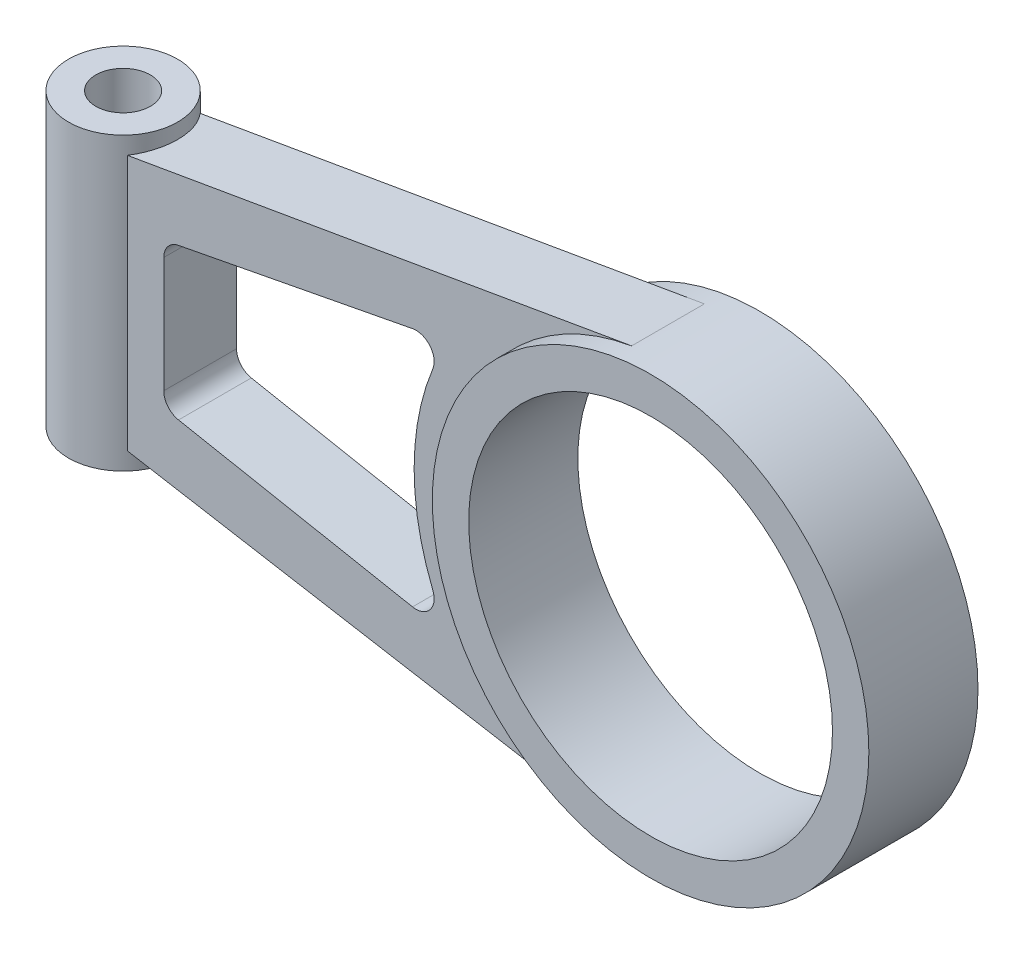
ISO-10303-21;
HEADER;
FILE_DESCRIPTION(('STEP AP214'),'2;1');
FILE_NAME('part.step','',(''),(''),'','','');
FILE_SCHEMA(('AUTOMOTIVE_DESIGN { 1 0 10303 214 1 1 1 1 }'));
ENDSEC;
DATA;
#1=APPLICATION_CONTEXT('core data for automotive mechanical design processes');
#2=APPLICATION_PROTOCOL_DEFINITION('international standard','automotive_design',2000,#1);
#3=PRODUCT_CONTEXT('',#1,'mechanical');
#4=PRODUCT('Part','Part','',(#3));
#5=PRODUCT_RELATED_PRODUCT_CATEGORY('part','',(#4));
#6=PRODUCT_DEFINITION_FORMATION('','',#4);
#7=PRODUCT_DEFINITION_CONTEXT('part definition',#1,'design');
#8=PRODUCT_DEFINITION('design','',#6,#7);
#9=PRODUCT_DEFINITION_SHAPE('','',#8);
#10=(LENGTH_UNIT() NAMED_UNIT(*) SI_UNIT(.MILLI.,.METRE.));
#11=(NAMED_UNIT(*) PLANE_ANGLE_UNIT() SI_UNIT($,.RADIAN.));
#12=(NAMED_UNIT(*) SI_UNIT($,.STERADIAN.) SOLID_ANGLE_UNIT());
#13=UNCERTAINTY_MEASURE_WITH_UNIT(LENGTH_MEASURE(1.E-05),#10,'distance_accuracy_value','');
#14=(GEOMETRIC_REPRESENTATION_CONTEXT(3) GLOBAL_UNCERTAINTY_ASSIGNED_CONTEXT((#13)) GLOBAL_UNIT_ASSIGNED_CONTEXT((#10,
#11,#12)) REPRESENTATION_CONTEXT('',''));
#15=CARTESIAN_POINT('',(0.,0.,0.));
#16=DIRECTION('',(0.,0.,1.));
#17=DIRECTION('',(1.,0.,0.));
#18=AXIS2_PLACEMENT_3D('',#15,#16,#17);
#19=CARTESIAN_POINT('',(0.,0.,10.));
#20=DIRECTION('',(0.,0.,1.));
#21=DIRECTION('',(1.,0.,0.));
#22=AXIS2_PLACEMENT_3D('',#19,#20,#21);
#23=PLANE('',#22);
#24=CARTESIAN_POINT('',(-133.819660112501,15.8679479378662,9.99999999999999));
#25=DIRECTION('',(0.,0.,1.));
#26=DIRECTION('',(1.,0.,0.));
#27=AXIS2_PLACEMENT_3D('',#24,#25,#26);
#28=CIRCLE('',#27,5.);
#29=CARTESIAN_POINT('',(-134.761592566539,20.77842278782,9.99999999999999));
#30=VERTEX_POINT('',#29);
#31=CARTESIAN_POINT('',(-138.819660112501,15.8679479378662,10.));
#32=VERTEX_POINT('',#31);
#33=EDGE_CURVE('E139',#30,#32,#28,.T.);
#34=ORIENTED_EDGE('',*,*,#33,.F.);
#35=DIRECTION('',(-0.982094969990767,-0.188386490807685,0.));
#36=VECTOR('',#35,1.);
#37=CARTESIAN_POINT('',(-8.62690465243416,44.9737113814315,10.));
#38=LINE('',#37,#36);
#39=CARTESIAN_POINT('',(-70.4355513802943,33.11751171192,9.99999999999999));
#40=VERTEX_POINT('',#39);
#41=EDGE_CURVE('E216',#40,#30,#38,.T.);
#42=ORIENTED_EDGE('',*,*,#41,.F.);
#43=CARTESIAN_POINT('',(-69.4936189262559,28.2070368619661,9.99999999999999));
#44=DIRECTION('',(0.,0.,1.));
#45=DIRECTION('',(1.,0.,0.));
#46=AXIS2_PLACEMENT_3D('',#43,#44,#45);
#47=CIRCLE('',#46,5.);
#48=CARTESIAN_POINT('',(-64.8607109978388,26.3265677378351,9.99999999999999));
#49=VERTEX_POINT('',#48);
#50=EDGE_CURVE('E217',#49,#40,#47,.T.);
#51=ORIENTED_EDGE('',*,*,#50,.F.);
#52=CARTESIAN_POINT('',(0.,0.,9.99999999999999));
#53=DIRECTION('',(0.,0.,1.));
#54=DIRECTION('',(1.,0.,0.));
#55=AXIS2_PLACEMENT_3D('',#52,#53,#54);
#56=CIRCLE('',#55,69.9999999999997);
#57=CARTESIAN_POINT('',(-64.8607109978386,-26.3265677378351,9.99999999999999));
#58=VERTEX_POINT('',#57);
#59=EDGE_CURVE('E219',#58,#49,#56,.F.);
#60=ORIENTED_EDGE('',*,*,#59,.F.);
#61=CARTESIAN_POINT('',(-69.4936189262554,-28.2070368619662,9.99999999999999));
#62=DIRECTION('',(0.,0.,1.));
#63=DIRECTION('',(1.,0.,0.));
#64=AXIS2_PLACEMENT_3D('',#61,#62,#63);
#65=CIRCLE('',#64,5.);
#66=CARTESIAN_POINT('',(-70.4355513802939,-33.11751171192,9.99999999999999));
#67=VERTEX_POINT('',#66);
#68=EDGE_CURVE('E225',#67,#58,#65,.T.);
#69=ORIENTED_EDGE('',*,*,#68,.F.);
#70=DIRECTION('',(0.982094969990768,-0.188386490807683,0.));
#71=VECTOR('',#70,1.);
#72=CARTESIAN_POINT('',(-8.62690465243404,-44.9737113814314,10.));
#73=LINE('',#72,#71);
#74=CARTESIAN_POINT('',(-134.761592566539,-20.7784227878201,9.99999999999999));
#75=VERTEX_POINT('',#74);
#76=EDGE_CURVE('E221',#75,#67,#73,.T.);
#77=ORIENTED_EDGE('',*,*,#76,.F.);
#78=CARTESIAN_POINT('',(-133.819660112501,-15.8679479378662,9.99999999999999));
#79=DIRECTION('',(0.,0.,1.));
#80=DIRECTION('',(1.,0.,0.));
#81=AXIS2_PLACEMENT_3D('',#78,#79,#80);
#82=CIRCLE('',#81,5.);
#83=CARTESIAN_POINT('',(-138.819660112501,-15.8679479378662,9.99999999999999));
#84=VERTEX_POINT('',#83);
#85=EDGE_CURVE('E226',#84,#75,#82,.T.);
#86=ORIENTED_EDGE('',*,*,#85,.F.);
#87=DIRECTION('',(0.,-1.,0.));
#88=VECTOR('',#87,1.);
#89=CARTESIAN_POINT('',(-138.819660112501,0.,10.));
#90=LINE('',#89,#88);
#91=EDGE_CURVE('E229',#32,#84,#90,.T.);
#92=ORIENTED_EDGE('',*,*,#91,.F.);
#93=EDGE_LOOP('',(#34,#42,#51,#60,#69,#77,#86,#92));
#94=FACE_BOUND('',#93,.T.);
#95=DIRECTION('',(-0.985406838508122,-0.170215635654975,0.));
#96=VECTOR('',#95,1.);
#97=CARTESIAN_POINT('',(-10.2129381392985,59.1244103104874,10.));
#98=LINE('',#97,#96);
#99=CARTESIAN_POINT('',(-10.2129381392985,59.1244103104874,10.));
#100=VERTEX_POINT('',#99);
#101=CARTESIAN_POINT('',(-148.819660112501,35.1819833201893,10.));
#102=VERTEX_POINT('',#101);
#103=EDGE_CURVE('E179',#100,#102,#98,.T.);
#104=ORIENTED_EDGE('',*,*,#103,.T.);
#105=DIRECTION('',(0.,-1.,0.));
#106=VECTOR('',#105,1.);
#107=CARTESIAN_POINT('',(-148.819660112501,40.,10.));
#108=LINE('',#107,#106);
#109=CARTESIAN_POINT('',(-148.819660112501,-35.1819833201894,10.));
#110=VERTEX_POINT('',#109);
#111=EDGE_CURVE('E188',#102,#110,#108,.T.);
#112=ORIENTED_EDGE('',*,*,#111,.T.);
#113=DIRECTION('',(-0.985406838508122,0.170215635654975,0.));
#114=VECTOR('',#113,1.);
#115=CARTESIAN_POINT('',(-10.2129381392985,-59.1244103104874,10.));
#116=LINE('',#115,#114);
#117=CARTESIAN_POINT('',(-10.2129381392985,-59.1244103104873,10.));
#118=VERTEX_POINT('',#117);
#119=EDGE_CURVE('E194',#118,#110,#116,.T.);
#120=ORIENTED_EDGE('',*,*,#119,.F.);
#121=CARTESIAN_POINT('',(0.,0.,10.));
#122=DIRECTION('',(0.,0.,1.));
#123=DIRECTION('',(1.,0.,0.));
#124=AXIS2_PLACEMENT_3D('',#121,#122,#123);
#125=CIRCLE('',#124,60.);
#126=EDGE_CURVE('E181',#100,#118,#125,.T.);
#127=ORIENTED_EDGE('',*,*,#126,.F.);
#128=EDGE_LOOP('',(#104,#112,#120,#127));
#129=FACE_BOUND('',#128,.T.);
#130=ADVANCED_FACE('F39',(#94,#129),#23,.T.);
#131=CARTESIAN_POINT('',(0.,0.,-10.));
#132=DIRECTION('',(0.,0.,1.));
#133=DIRECTION('',(1.,0.,0.));
#134=AXIS2_PLACEMENT_3D('',#131,#132,#133);
#135=PLANE('',#134);
#136=DIRECTION('',(-0.982094969990767,-0.188386490807685,0.));
#137=VECTOR('',#136,1.);
#138=CARTESIAN_POINT('',(-8.62690465243416,44.9737113814315,-10.));
#139=LINE('',#138,#137);
#140=CARTESIAN_POINT('',(-70.4355513802943,33.11751171192,-9.99999999999999));
#141=VERTEX_POINT('',#140);
#142=CARTESIAN_POINT('',(-134.761592566539,20.77842278782,-9.99999999999999));
#143=VERTEX_POINT('',#142);
#144=EDGE_CURVE('E50',#141,#143,#139,.T.);
#145=ORIENTED_EDGE('',*,*,#144,.T.);
#146=CARTESIAN_POINT('',(-133.819660112501,15.8679479378662,-9.99999999999999));
#147=DIRECTION('',(0.,0.,1.));
#148=DIRECTION('',(1.,0.,0.));
#149=AXIS2_PLACEMENT_3D('',#146,#147,#148);
#150=CIRCLE('',#149,5.);
#151=CARTESIAN_POINT('',(-138.819660112501,15.8679479378662,-9.99999999999999));
#152=VERTEX_POINT('',#151);
#153=EDGE_CURVE('E11',#143,#152,#150,.T.);
#154=ORIENTED_EDGE('',*,*,#153,.T.);
#155=DIRECTION('',(0.,-1.,0.));
#156=VECTOR('',#155,1.);
#157=CARTESIAN_POINT('',(-138.819660112501,0.,-10.));
#158=LINE('',#157,#156);
#159=CARTESIAN_POINT('',(-138.819660112501,-15.8679479378662,-10.));
#160=VERTEX_POINT('',#159);
#161=EDGE_CURVE('E123',#152,#160,#158,.T.);
#162=ORIENTED_EDGE('',*,*,#161,.T.);
#163=CARTESIAN_POINT('',(-133.819660112501,-15.8679479378662,-9.99999999999999));
#164=DIRECTION('',(0.,0.,1.));
#165=DIRECTION('',(1.,0.,0.));
#166=AXIS2_PLACEMENT_3D('',#163,#164,#165);
#167=CIRCLE('',#166,5.);
#168=CARTESIAN_POINT('',(-134.761592566539,-20.7784227878201,-9.99999999999999));
#169=VERTEX_POINT('',#168);
#170=EDGE_CURVE('E129',#160,#169,#167,.T.);
#171=ORIENTED_EDGE('',*,*,#170,.T.);
#172=DIRECTION('',(0.982094969990768,-0.188386490807683,0.));
#173=VECTOR('',#172,1.);
#174=CARTESIAN_POINT('',(-8.62690465243404,-44.9737113814314,-10.));
#175=LINE('',#174,#173);
#176=CARTESIAN_POINT('',(-70.4355513802939,-33.11751171192,-9.99999999999999));
#177=VERTEX_POINT('',#176);
#178=EDGE_CURVE('E156',#169,#177,#175,.T.);
#179=ORIENTED_EDGE('',*,*,#178,.T.);
#180=CARTESIAN_POINT('',(-69.4936189262554,-28.2070368619662,-9.99999999999999));
#181=DIRECTION('',(0.,0.,1.));
#182=DIRECTION('',(1.,0.,0.));
#183=AXIS2_PLACEMENT_3D('',#180,#181,#182);
#184=CIRCLE('',#183,5.);
#185=CARTESIAN_POINT('',(-64.8607109978386,-26.3265677378351,-9.99999999999999));
#186=VERTEX_POINT('',#185);
#187=EDGE_CURVE('E153',#177,#186,#184,.T.);
#188=ORIENTED_EDGE('',*,*,#187,.T.);
#189=CARTESIAN_POINT('',(0.,0.,-9.99999999999999));
#190=DIRECTION('',(0.,0.,1.));
#191=DIRECTION('',(1.,0.,0.));
#192=AXIS2_PLACEMENT_3D('',#189,#190,#191);
#193=CIRCLE('',#192,69.9999999999997);
#194=CARTESIAN_POINT('',(-64.8607109978388,26.3265677378351,-9.99999999999999));
#195=VERTEX_POINT('',#194);
#196=EDGE_CURVE('E149',#186,#195,#193,.F.);
#197=ORIENTED_EDGE('',*,*,#196,.T.);
#198=CARTESIAN_POINT('',(-69.4936189262559,28.2070368619661,-9.99999999999999));
#199=DIRECTION('',(0.,0.,1.));
#200=DIRECTION('',(1.,0.,0.));
#201=AXIS2_PLACEMENT_3D('',#198,#199,#200);
#202=CIRCLE('',#201,5.);
#203=EDGE_CURVE('E144',#195,#141,#202,.T.);
#204=ORIENTED_EDGE('',*,*,#203,.T.);
#205=EDGE_LOOP('',(#145,#154,#162,#171,#179,#188,#197,#204));
#206=FACE_BOUND('',#205,.T.);
#207=DIRECTION('',(0.,-1.,0.));
#208=VECTOR('',#207,1.);
#209=CARTESIAN_POINT('',(-148.819660112501,40.,-10.));
#210=LINE('',#209,#208);
#211=CARTESIAN_POINT('',(-148.819660112501,35.1819833201893,-10.));
#212=VERTEX_POINT('',#211);
#213=CARTESIAN_POINT('',(-148.819660112501,-35.1819833201894,-10.));
#214=VERTEX_POINT('',#213);
#215=EDGE_CURVE('E128',#212,#214,#210,.T.);
#216=ORIENTED_EDGE('',*,*,#215,.F.);
#217=DIRECTION('',(-0.985406838508122,-0.170215635654975,0.));
#218=VECTOR('',#217,1.);
#219=CARTESIAN_POINT('',(-10.2129381392985,59.1244103104874,-10.));
#220=LINE('',#219,#218);
#221=CARTESIAN_POINT('',(-10.2129381392985,59.1244103104873,-10.));
#222=VERTEX_POINT('',#221);
#223=EDGE_CURVE('E178',#222,#212,#220,.T.);
#224=ORIENTED_EDGE('',*,*,#223,.F.);
#225=CARTESIAN_POINT('',(0.,0.,-10.));
#226=DIRECTION('',(0.,0.,1.));
#227=DIRECTION('',(1.,0.,0.));
#228=AXIS2_PLACEMENT_3D('',#225,#226,#227);
#229=CIRCLE('',#228,60.);
#230=CARTESIAN_POINT('',(-10.2129381392985,-59.1244103104874,-10.));
#231=VERTEX_POINT('',#230);
#232=EDGE_CURVE('E186',#222,#231,#229,.T.);
#233=ORIENTED_EDGE('',*,*,#232,.T.);
#234=DIRECTION('',(-0.985406838508122,0.170215635654975,0.));
#235=VECTOR('',#234,1.);
#236=CARTESIAN_POINT('',(-10.2129381392985,-59.1244103104874,-10.));
#237=LINE('',#236,#235);
#238=EDGE_CURVE('E184',#231,#214,#237,.T.);
#239=ORIENTED_EDGE('',*,*,#238,.T.);
#240=EDGE_LOOP('',(#216,#224,#233,#239));
#241=FACE_BOUND('',#240,.T.);
#242=ADVANCED_FACE('F143',(#206,#241),#135,.F.);
#243=CARTESIAN_POINT('',(0.,0.,15.));
#244=DIRECTION('',(0.,0.,1.));
#245=DIRECTION('',(1.,0.,0.));
#246=AXIS2_PLACEMENT_3D('',#243,#244,#245);
#247=PLANE('',#246);
#248=CARTESIAN_POINT('',(0.,0.,15.));
#249=DIRECTION('',(0.,0.,1.));
#250=DIRECTION('',(1.,0.,0.));
#251=AXIS2_PLACEMENT_3D('',#248,#249,#250);
#252=CIRCLE('',#251,60.);
#253=CARTESIAN_POINT('',(60.,0.,15.));
#254=VERTEX_POINT('',#253);
#255=EDGE_CURVE('E165',#254,#254,#252,.T.);
#256=ORIENTED_EDGE('',*,*,#255,.T.);
#257=EDGE_LOOP('',(#256));
#258=FACE_BOUND('',#257,.T.);
#259=CARTESIAN_POINT('',(0.,0.,15.));
#260=DIRECTION('',(0.,0.,1.));
#261=DIRECTION('',(1.,0.,0.));
#262=AXIS2_PLACEMENT_3D('',#259,#260,#261);
#263=CIRCLE('',#262,50.);
#264=CARTESIAN_POINT('',(50.,0.,15.));
#265=VERTEX_POINT('',#264);
#266=EDGE_CURVE('E167',#265,#265,#263,.T.);
#267=ORIENTED_EDGE('',*,*,#266,.F.);
#268=EDGE_LOOP('',(#267));
#269=FACE_BOUND('',#268,.T.);
#270=ADVANCED_FACE('F283',(#258,#269),#247,.T.);
#271=CARTESIAN_POINT('',(0.,0.,-15.));
#272=DIRECTION('',(0.,0.,1.));
#273=DIRECTION('',(1.,0.,0.));
#274=AXIS2_PLACEMENT_3D('',#271,#272,#273);
#275=PLANE('',#274);
#276=CARTESIAN_POINT('',(0.,0.,-15.));
#277=DIRECTION('',(0.,0.,1.));
#278=DIRECTION('',(1.,0.,0.));
#279=AXIS2_PLACEMENT_3D('',#276,#277,#278);
#280=CIRCLE('',#279,60.);
#281=CARTESIAN_POINT('',(60.,0.,-15.));
#282=VERTEX_POINT('',#281);
#283=EDGE_CURVE('E162',#282,#282,#280,.T.);
#284=ORIENTED_EDGE('',*,*,#283,.F.);
#285=EDGE_LOOP('',(#284));
#286=FACE_BOUND('',#285,.T.);
#287=CARTESIAN_POINT('',(0.,0.,-15.));
#288=DIRECTION('',(0.,0.,1.));
#289=DIRECTION('',(1.,0.,0.));
#290=AXIS2_PLACEMENT_3D('',#287,#288,#289);
#291=CIRCLE('',#290,50.);
#292=CARTESIAN_POINT('',(50.,0.,-15.));
#293=VERTEX_POINT('',#292);
#294=EDGE_CURVE('E166',#293,#293,#291,.T.);
#295=ORIENTED_EDGE('',*,*,#294,.T.);
#296=EDGE_LOOP('',(#295));
#297=FACE_BOUND('',#296,.T.);
#298=ADVANCED_FACE('F301',(#286,#297),#275,.F.);
#299=CARTESIAN_POINT('',(0.,0.,15.));
#300=DIRECTION('',(0.,0.,-1.));
#301=DIRECTION('',(-1.,0.,0.));
#302=AXIS2_PLACEMENT_3D('',#299,#300,#301);
#303=CYLINDRICAL_SURFACE('',#302,60.);
#304=DIRECTION('',(0.,0.,-1.));
#305=VECTOR('',#304,1.);
#306=CARTESIAN_POINT('',(-10.2129381392985,59.1244103104874,10.));
#307=LINE('',#306,#305);
#308=EDGE_CURVE('E172',#100,#222,#307,.T.);
#309=ORIENTED_EDGE('',*,*,#308,.F.);
#310=ORIENTED_EDGE('',*,*,#126,.T.);
#311=DIRECTION('',(0.,0.,-1.));
#312=VECTOR('',#311,1.);
#313=CARTESIAN_POINT('',(-10.2129381392985,-59.1244103104874,10.));
#314=LINE('',#313,#312);
#315=EDGE_CURVE('E175',#118,#231,#314,.T.);
#316=ORIENTED_EDGE('',*,*,#315,.T.);
#317=ORIENTED_EDGE('',*,*,#232,.F.);
#318=EDGE_LOOP('',(#309,#310,#316,#317));
#319=FACE_BOUND('',#318,.T.);
#320=ORIENTED_EDGE('',*,*,#255,.F.);
#321=EDGE_LOOP('',(#320));
#322=FACE_BOUND('',#321,.T.);
#323=ORIENTED_EDGE('',*,*,#283,.T.);
#324=EDGE_LOOP('',(#323));
#325=FACE_BOUND('',#324,.T.);
#326=ADVANCED_FACE('F41',(#319,#322,#325),#303,.T.);
#327=CARTESIAN_POINT('',(0.,0.,15.));
#328=DIRECTION('',(0.,0.,-1.));
#329=DIRECTION('',(-1.,0.,0.));
#330=AXIS2_PLACEMENT_3D('',#327,#328,#329);
#331=CYLINDRICAL_SURFACE('',#330,50.);
#332=ORIENTED_EDGE('',*,*,#266,.T.);
#333=EDGE_LOOP('',(#332));
#334=FACE_BOUND('',#333,.T.);
#335=ORIENTED_EDGE('',*,*,#294,.F.);
#336=EDGE_LOOP('',(#335));
#337=FACE_BOUND('',#336,.T.);
#338=ADVANCED_FACE('F294',(#334,#337),#331,.F.);
#339=CARTESIAN_POINT('',(-10.2129381392985,59.1244103104874,10.));
#340=DIRECTION('',(0.170215635654975,-0.985406838508122,0.));
#341=DIRECTION('',(0.985406838508122,0.170215635654975,0.));
#342=AXIS2_PLACEMENT_3D('',#339,#340,#341);
#343=PLANE('',#342);
#344=CARTESIAN_POINT('',(-160.,33.250731591035,0.));
#345=DIRECTION('',(0.170215635654975,-0.985406838508122,0.));
#346=DIRECTION('',(-0.985406838508122,-0.170215635654975,0.));
#347=AXIS2_PLACEMENT_3D('',#344,#345,#346);
#348=ELLIPSE('',#347,15.2221391346437,15.);
#349=EDGE_CURVE('E197',#102,#212,#348,.F.);
#350=ORIENTED_EDGE('',*,*,#349,.F.);
#351=ORIENTED_EDGE('',*,*,#103,.F.);
#352=ORIENTED_EDGE('',*,*,#308,.T.);
#353=ORIENTED_EDGE('',*,*,#223,.T.);
#354=EDGE_LOOP('',(#350,#351,#352,#353));
#355=FACE_BOUND('',#354,.T.);
#356=ADVANCED_FACE('F288',(#355),#343,.F.);
#357=CARTESIAN_POINT('',(-10.2129381392985,-59.1244103104874,10.));
#358=DIRECTION('',(-0.170215635654975,-0.985406838508122,0.));
#359=DIRECTION('',(0.985406838508123,-0.170215635654975,0.));
#360=AXIS2_PLACEMENT_3D('',#357,#358,#359);
#361=PLANE('',#360);
#362=ORIENTED_EDGE('',*,*,#119,.T.);
#363=CARTESIAN_POINT('',(-160.,-33.2507315910351,0.));
#364=DIRECTION('',(-0.170215635654975,-0.985406838508122,0.));
#365=DIRECTION('',(0.985406838508123,-0.170215635654975,0.));
#366=AXIS2_PLACEMENT_3D('',#363,#364,#365);
#367=ELLIPSE('',#366,15.2221391346437,15.);
#368=EDGE_CURVE('E199',#110,#214,#367,.F.);
#369=ORIENTED_EDGE('',*,*,#368,.T.);
#370=ORIENTED_EDGE('',*,*,#238,.F.);
#371=ORIENTED_EDGE('',*,*,#315,.F.);
#372=EDGE_LOOP('',(#362,#369,#370,#371));
#373=FACE_BOUND('',#372,.T.);
#374=ADVANCED_FACE('F291',(#373),#361,.T.);
#375=CARTESIAN_POINT('',(-160.,40.,0.));
#376=DIRECTION('',(0.,1.,0.));
#377=DIRECTION('',(0.,0.,1.));
#378=AXIS2_PLACEMENT_3D('',#375,#376,#377);
#379=PLANE('',#378);
#380=CARTESIAN_POINT('',(-160.,40.,0.));
#381=DIRECTION('',(0.,1.,0.));
#382=DIRECTION('',(0.,0.,1.));
#383=AXIS2_PLACEMENT_3D('',#380,#381,#382);
#384=CIRCLE('',#383,15.);
#385=CARTESIAN_POINT('',(-160.,40.,15.));
#386=VERTEX_POINT('',#385);
#387=EDGE_CURVE('E201',#386,#386,#384,.T.);
#388=ORIENTED_EDGE('',*,*,#387,.T.);
#389=EDGE_LOOP('',(#388));
#390=FACE_BOUND('',#389,.T.);
#391=CARTESIAN_POINT('',(-160.,40.,0.));
#392=DIRECTION('',(0.,1.,0.));
#393=DIRECTION('',(0.,0.,1.));
#394=AXIS2_PLACEMENT_3D('',#391,#392,#393);
#395=CIRCLE('',#394,7.50000000000001);
#396=CARTESIAN_POINT('',(-160.,40.,7.50000000000001));
#397=VERTEX_POINT('',#396);
#398=EDGE_CURVE('E210',#397,#397,#395,.T.);
#399=ORIENTED_EDGE('',*,*,#398,.F.);
#400=EDGE_LOOP('',(#399));
#401=FACE_BOUND('',#400,.T.);
#402=ADVANCED_FACE('F299',(#390,#401),#379,.T.);
#403=CARTESIAN_POINT('',(-160.,-40.,0.));
#404=DIRECTION('',(0.,1.,0.));
#405=DIRECTION('',(0.,0.,1.));
#406=AXIS2_PLACEMENT_3D('',#403,#404,#405);
#407=PLANE('',#406);
#408=CARTESIAN_POINT('',(-160.,-40.,0.));
#409=DIRECTION('',(0.,1.,0.));
#410=DIRECTION('',(0.,0.,1.));
#411=AXIS2_PLACEMENT_3D('',#408,#409,#410);
#412=CIRCLE('',#411,15.);
#413=CARTESIAN_POINT('',(-160.,-40.,15.));
#414=VERTEX_POINT('',#413);
#415=EDGE_CURVE('E204',#414,#414,#412,.T.);
#416=ORIENTED_EDGE('',*,*,#415,.F.);
#417=EDGE_LOOP('',(#416));
#418=FACE_BOUND('',#417,.T.);
#419=CARTESIAN_POINT('',(-160.,-40.,0.));
#420=DIRECTION('',(0.,1.,0.));
#421=DIRECTION('',(0.,0.,1.));
#422=AXIS2_PLACEMENT_3D('',#419,#420,#421);
#423=CIRCLE('',#422,7.50000000000001);
#424=CARTESIAN_POINT('',(-160.,-40.,7.50000000000001));
#425=VERTEX_POINT('',#424);
#426=EDGE_CURVE('E209',#425,#425,#423,.T.);
#427=ORIENTED_EDGE('',*,*,#426,.T.);
#428=EDGE_LOOP('',(#427));
#429=FACE_BOUND('',#428,.T.);
#430=ADVANCED_FACE('F331',(#418,#429),#407,.F.);
#431=CARTESIAN_POINT('',(-160.,40.,0.));
#432=DIRECTION('',(0.,-1.,0.));
#433=DIRECTION('',(0.,0.,-1.));
#434=AXIS2_PLACEMENT_3D('',#431,#432,#433);
#435=CYLINDRICAL_SURFACE('',#434,15.);
#436=ORIENTED_EDGE('',*,*,#111,.F.);
#437=ORIENTED_EDGE('',*,*,#349,.T.);
#438=ORIENTED_EDGE('',*,*,#215,.T.);
#439=ORIENTED_EDGE('',*,*,#368,.F.);
#440=EDGE_LOOP('',(#436,#437,#438,#439));
#441=FACE_BOUND('',#440,.T.);
#442=ORIENTED_EDGE('',*,*,#387,.F.);
#443=EDGE_LOOP('',(#442));
#444=FACE_BOUND('',#443,.T.);
#445=ORIENTED_EDGE('',*,*,#415,.T.);
#446=EDGE_LOOP('',(#445));
#447=FACE_BOUND('',#446,.T.);
#448=ADVANCED_FACE('F289',(#441,#444,#447),#435,.T.);
#449=CARTESIAN_POINT('',(-160.,40.,0.));
#450=DIRECTION('',(0.,-1.,0.));
#451=DIRECTION('',(0.,0.,-1.));
#452=AXIS2_PLACEMENT_3D('',#449,#450,#451);
#453=CYLINDRICAL_SURFACE('',#452,7.50000000000001);
#454=ORIENTED_EDGE('',*,*,#398,.T.);
#455=EDGE_LOOP('',(#454));
#456=FACE_BOUND('',#455,.T.);
#457=ORIENTED_EDGE('',*,*,#426,.F.);
#458=EDGE_LOOP('',(#457));
#459=FACE_BOUND('',#458,.T.);
#460=ADVANCED_FACE('F277',(#456,#459),#453,.F.);
#461=CARTESIAN_POINT('',(-133.819660112501,15.8679479378662,-42.5));
#462=DIRECTION('',(0.,0.,1.));
#463=DIRECTION('',(1.,0.,0.));
#464=AXIS2_PLACEMENT_3D('',#461,#462,#463);
#465=CYLINDRICAL_SURFACE('',#464,5.);
#466=ORIENTED_EDGE('',*,*,#33,.T.);
#467=DIRECTION('',(0.,0.,1.));
#468=VECTOR('',#467,1.);
#469=CARTESIAN_POINT('',(-138.819660112501,15.8679479378662,-42.5));
#470=LINE('',#469,#468);
#471=EDGE_CURVE('E53',#152,#32,#470,.T.);
#472=ORIENTED_EDGE('',*,*,#471,.F.);
#473=ORIENTED_EDGE('',*,*,#153,.F.);
#474=DIRECTION('',(0.,0.,1.));
#475=VECTOR('',#474,1.);
#476=CARTESIAN_POINT('',(-134.761592566539,20.77842278782,-42.5));
#477=LINE('',#476,#475);
#478=EDGE_CURVE('E228',#143,#30,#477,.T.);
#479=ORIENTED_EDGE('',*,*,#478,.T.);
#480=EDGE_LOOP('',(#466,#472,#473,#479));
#481=FACE_BOUND('',#480,.T.);
#482=ADVANCED_FACE('F134',(#481),#465,.F.);
#483=CARTESIAN_POINT('',(-134.761592566539,20.77842278782,-42.5));
#484=DIRECTION('',(-0.188386490807685,0.982094969990767,0.));
#485=DIRECTION('',(-0.982094969990767,-0.188386490807685,0.));
#486=AXIS2_PLACEMENT_3D('',#483,#484,#485);
#487=PLANE('',#486);
#488=ORIENTED_EDGE('',*,*,#41,.T.);
#489=ORIENTED_EDGE('',*,*,#478,.F.);
#490=ORIENTED_EDGE('',*,*,#144,.F.);
#491=DIRECTION('',(0.,0.,1.));
#492=VECTOR('',#491,1.);
#493=CARTESIAN_POINT('',(-70.4355513802943,33.11751171192,-42.5));
#494=LINE('',#493,#492);
#495=EDGE_CURVE('E243',#141,#40,#494,.T.);
#496=ORIENTED_EDGE('',*,*,#495,.T.);
#497=EDGE_LOOP('',(#488,#489,#490,#496));
#498=FACE_BOUND('',#497,.T.);
#499=ADVANCED_FACE('F268',(#498),#487,.F.);
#500=CARTESIAN_POINT('',(-69.4936189262559,28.2070368619661,-42.5));
#501=DIRECTION('',(0.,0.,1.));
#502=DIRECTION('',(1.,0.,0.));
#503=AXIS2_PLACEMENT_3D('',#500,#501,#502);
#504=CYLINDRICAL_SURFACE('',#503,5.);
#505=ORIENTED_EDGE('',*,*,#50,.T.);
#506=ORIENTED_EDGE('',*,*,#495,.F.);
#507=ORIENTED_EDGE('',*,*,#203,.F.);
#508=DIRECTION('',(0.,0.,1.));
#509=VECTOR('',#508,1.);
#510=CARTESIAN_POINT('',(-64.8607109978388,26.3265677378351,-42.5));
#511=LINE('',#510,#509);
#512=EDGE_CURVE('E241',#195,#49,#511,.T.);
#513=ORIENTED_EDGE('',*,*,#512,.T.);
#514=EDGE_LOOP('',(#505,#506,#507,#513));
#515=FACE_BOUND('',#514,.T.);
#516=ADVANCED_FACE('F270',(#515),#504,.F.);
#517=CARTESIAN_POINT('',(0.,0.,-42.5));
#518=DIRECTION('',(0.,0.,1.));
#519=DIRECTION('',(1.,0.,0.));
#520=AXIS2_PLACEMENT_3D('',#517,#518,#519);
#521=CYLINDRICAL_SURFACE('',#520,69.9999999999997);
#522=ORIENTED_EDGE('',*,*,#59,.T.);
#523=ORIENTED_EDGE('',*,*,#512,.F.);
#524=ORIENTED_EDGE('',*,*,#196,.F.);
#525=DIRECTION('',(0.,0.,1.));
#526=VECTOR('',#525,1.);
#527=CARTESIAN_POINT('',(-64.8607109978386,-26.3265677378351,-42.5));
#528=LINE('',#527,#526);
#529=EDGE_CURVE('E236',#186,#58,#528,.T.);
#530=ORIENTED_EDGE('',*,*,#529,.T.);
#531=EDGE_LOOP('',(#522,#523,#524,#530));
#532=FACE_BOUND('',#531,.T.);
#533=ADVANCED_FACE('F264',(#532),#521,.T.);
#534=CARTESIAN_POINT('',(-69.4936189262554,-28.2070368619662,-42.5));
#535=DIRECTION('',(0.,0.,1.));
#536=DIRECTION('',(1.,0.,0.));
#537=AXIS2_PLACEMENT_3D('',#534,#535,#536);
#538=CYLINDRICAL_SURFACE('',#537,5.);
#539=ORIENTED_EDGE('',*,*,#68,.T.);
#540=ORIENTED_EDGE('',*,*,#529,.F.);
#541=ORIENTED_EDGE('',*,*,#187,.F.);
#542=DIRECTION('',(0.,0.,1.));
#543=VECTOR('',#542,1.);
#544=CARTESIAN_POINT('',(-70.4355513802939,-33.11751171192,-42.5));
#545=LINE('',#544,#543);
#546=EDGE_CURVE('E233',#177,#67,#545,.T.);
#547=ORIENTED_EDGE('',*,*,#546,.T.);
#548=EDGE_LOOP('',(#539,#540,#541,#547));
#549=FACE_BOUND('',#548,.T.);
#550=ADVANCED_FACE('F257',(#549),#538,.F.);
#551=CARTESIAN_POINT('',(-134.761592566539,-20.7784227878201,-42.5));
#552=DIRECTION('',(-0.188386490807683,-0.982094969990768,0.));
#553=DIRECTION('',(0.982094969990768,-0.188386490807683,0.));
#554=AXIS2_PLACEMENT_3D('',#551,#552,#553);
#555=PLANE('',#554);
#556=ORIENTED_EDGE('',*,*,#76,.T.);
#557=ORIENTED_EDGE('',*,*,#546,.F.);
#558=ORIENTED_EDGE('',*,*,#178,.F.);
#559=DIRECTION('',(0.,0.,1.));
#560=VECTOR('',#559,1.);
#561=CARTESIAN_POINT('',(-134.761592566539,-20.7784227878201,-42.5));
#562=LINE('',#561,#560);
#563=EDGE_CURVE('E234',#169,#75,#562,.T.);
#564=ORIENTED_EDGE('',*,*,#563,.T.);
#565=EDGE_LOOP('',(#556,#557,#558,#564));
#566=FACE_BOUND('',#565,.T.);
#567=ADVANCED_FACE('F260',(#566),#555,.F.);
#568=CARTESIAN_POINT('',(-133.819660112501,-15.8679479378662,-42.5));
#569=DIRECTION('',(0.,0.,1.));
#570=DIRECTION('',(1.,0.,0.));
#571=AXIS2_PLACEMENT_3D('',#568,#569,#570);
#572=CYLINDRICAL_SURFACE('',#571,5.);
#573=ORIENTED_EDGE('',*,*,#85,.T.);
#574=ORIENTED_EDGE('',*,*,#563,.F.);
#575=ORIENTED_EDGE('',*,*,#170,.F.);
#576=DIRECTION('',(0.,0.,1.));
#577=VECTOR('',#576,1.);
#578=CARTESIAN_POINT('',(-138.819660112501,-15.8679479378662,-42.5));
#579=LINE('',#578,#577);
#580=EDGE_CURVE('E56',#160,#84,#579,.T.);
#581=ORIENTED_EDGE('',*,*,#580,.T.);
#582=EDGE_LOOP('',(#573,#574,#575,#581));
#583=FACE_BOUND('',#582,.T.);
#584=ADVANCED_FACE('F251',(#583),#572,.F.);
#585=CARTESIAN_POINT('',(-138.819660112501,15.8679479378662,-42.5));
#586=DIRECTION('',(-1.,0.,0.));
#587=DIRECTION('',(0.,0.,1.));
#588=AXIS2_PLACEMENT_3D('',#585,#586,#587);
#589=PLANE('',#588);
#590=ORIENTED_EDGE('',*,*,#91,.T.);
#591=ORIENTED_EDGE('',*,*,#580,.F.);
#592=ORIENTED_EDGE('',*,*,#161,.F.);
#593=ORIENTED_EDGE('',*,*,#471,.T.);
#594=EDGE_LOOP('',(#590,#591,#592,#593));
#595=FACE_BOUND('',#594,.T.);
#596=ADVANCED_FACE('F127',(#595),#589,.F.);
#597=CLOSED_SHELL('',(#130,#242,#270,#298,#326,#338,#356,#374,#402,#430,#448,#460,#482,#499,
#516,#533,#550,#567,#584,#596));
#598=MANIFOLD_SOLID_BREP('B2',#597);
#599=ADVANCED_BREP_SHAPE_REPRESENTATION('',(#18,#598),#14);
#600=SHAPE_DEFINITION_REPRESENTATION(#9,#599);
ENDSEC;
END-ISO-10303-21;
